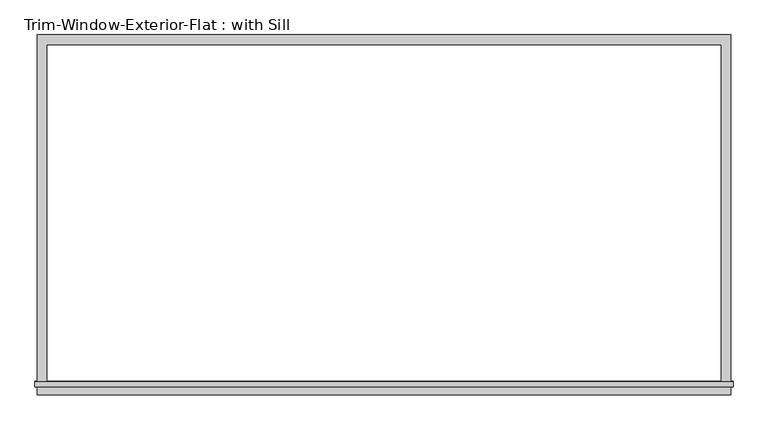
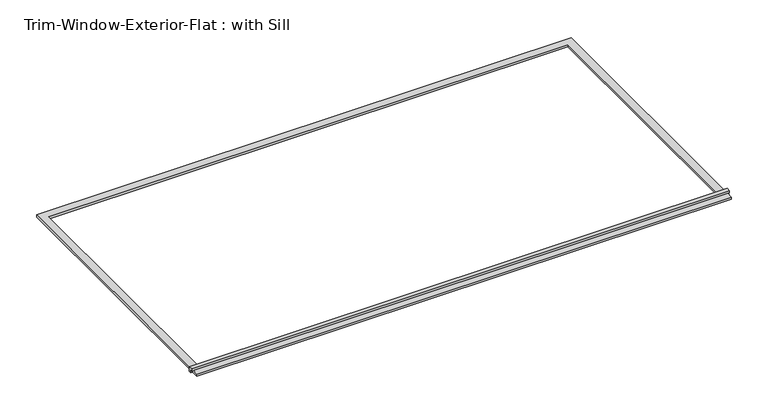
"""IFC4 building model written with IfcOpenShell, lengths in millimetres: proxy geometry, Trim-Window-Exterior-Flat : with Sill."""

from ifc_helpers import new_model, si_unit, frame, origin, origin_with_axes, place, context, project, spatial, polyline, outline, extrude, source, transform, mapped, element, save


def trim_window_exterior_flat_with_sill_170b7f0e(model_context):
    return source(origin(), model_context, "Body", "SweptSolid", [
        extrude(outline(polyline([(2038.35, -2003.3823709), (2038.35, -2060.5323709), (-2038.35, -2060.5323709), (-2038.35, -2003.3823709), (2038.35, -2003.3823709)])), origin_with_axes(), (0.0, 0.0, 1.0), 19.05),
        extrude(outline(polyline([(-2012.95, 38.1), (-1983.6580645, 38.1), (-1981.2, 19.05), (-1981.2, 0.0), (-2003.3823709, 0.0), (-2003.3823709, 19.05), (-2012.95, 19.05), (-2012.95, 38.1)])), frame((-2051.05, 0.0, 0.0), z_axis=(1.0, 0.0, 0.0), x_axis=(0.0, 1.0, 0.0)), (0.0, 0.0, 1.0), 4102.1),
        extrude(outline(polyline([(-2038.35, 57.15), (2038.35, 57.15), (2038.35, -1981.2), (1981.2, -1981.2), (1981.2, 0.0), (-1981.2, 0.0), (-1981.2, -1981.2), (-2038.35, -1981.2), (-2038.35, 57.15)])), origin_with_axes(), (0.0, 0.0, 1.0), 19.05),
    ])


if __name__ == "__main__":
    model = new_model("IFC4")
    model_context = context("Model", 3, world=origin())
    ifc_project = project(units=[si_unit("LENGTHUNIT", "METRE", prefix="MILLI")], contexts=[model_context])
    site = spatial("IfcSite", under=ifc_project)
    building = spatial("IfcBuilding", under=site)
    placement = place(None, origin())
    trim_window_exterior_flat_with_sill_shape = trim_window_exterior_flat_with_sill_170b7f0e(model_context)
    element("IfcBuildingElementProxy", 1, Name="Trim-Window-Exterior-Flat : with Sill", ObjectType="Trim-Window-Exterior-Flat : with Sill", at=placement, inside=building, context=model_context, shape_type="MappedRepresentation", body=[
        mapped(trim_window_exterior_flat_with_sill_shape, transform((0.0, 0.0, 0.0), x_axis=(1.0, 0.0, 0.0), y_axis=(0.0, 1.0, 0.0), z_axis=(0.0, 0.0, 1.0))),
    ])
    save(model, "model.ifc")

# Revit data of these elements
# Type "Trim-Window-Exterior-Flat : with Sill"
#   Trim Width = 0.1875 ft
#   Trim Thickness_Picture Frame = 0.104167 ft
#   Trim Thickness_with Sill = 0.0625 ft
#   Sill Thickness = 0.104167 ft
#   Opening Width [instance default] = 2 ft
#   Opening Height [instance default] = 3 ft
#   Default Elevation = 4 ft
#   Sill = yes
#   Picture Frame = no
#   Trim Material [instance default] = none
# Element 1 (IfcBuildingElementProxy, "Trim-Window-Exterior-Flat : with Sill")
#   Opening Width = 13 ft
#   Opening Height = 6.5 ft
#   Trim Material = Clad - White
#   Materials on its faces: "Clad - White"
# Materials
#   "Clad - White": class "Wood", colour RGB 242 242 238, transparency 0, Cost = 0
